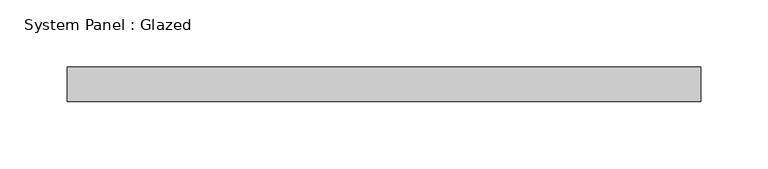
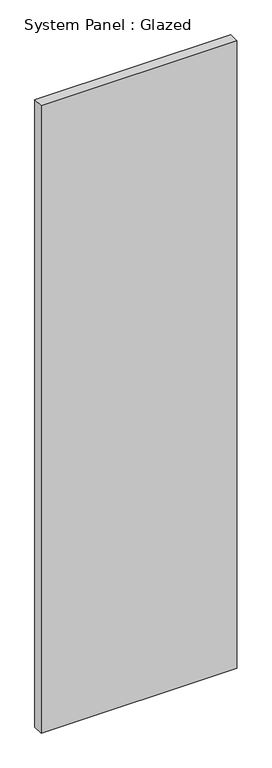
"""IFC4 building model written with IfcOpenShell, lengths in millimetres: plate geometry, System Panel : Glazed."""

from ifc_helpers import new_model, si_unit, origin, origin_with_axes, place, context, project, spatial, polyline, outline, extrude, source, transform, mapped, element, save


def system_panel_glazed_7060130a(model_context):
    return source(origin(), model_context, "Body", "SweptSolid", [
        extrude(outline(polyline([(234.95, 19.05), (-234.95, 19.05), (-234.95, 44.45), (234.95, 44.45), (234.95, 19.05)])), origin_with_axes(), (0.0, 0.0, 1.0), 1592.9882445),
    ])


if __name__ == "__main__":
    model = new_model("IFC4")
    model_context = context("Model", 3, world=origin())
    ifc_project = project(units=[si_unit("LENGTHUNIT", "METRE", prefix="MILLI")], contexts=[model_context])
    site = spatial("IfcSite", under=ifc_project)
    building = spatial("IfcBuilding", under=site)
    placement = place(None, origin())
    system_panel_glazed_shape = system_panel_glazed_7060130a(model_context)
    element("IfcPlate", 1, ObjectType="System Panel : Glazed", at=placement, inside=building, context=model_context, shape_type="MappedRepresentation", body=[
        mapped(system_panel_glazed_shape, transform((0.0, 0.0, 0.0), x_axis=(1.0, 0.0, 0.0), y_axis=(0.0, 1.0, 0.0), z_axis=(0.0, 0.0, 1.0))),
    ])
    save(model, "model.ifc")

# Revit data of these elements
# Type "System Panel : Glazed"
#   Construction Type Id = "GSP4R"
#   Analytic Construction = "1/8 in Pilkington single glazing"
#   Visual Light Transmittance = 0.9
#   Solar Heat Gain Coefficient = 0.86
#   Heat Transfer Coefficient (U) = 1.18115 BTU/(h·ft²·°F)
#   Define Thermal Properties by = 1
# Element 1 (IfcPlate, "System Panel : Glazed")
#   Materials on its faces: "Glass"
# Materials
#   "Glass": class "Glass", colour RGB 0 128 192, transparency 0.75, Description = "Soda Lime Glass", Cost = 0
